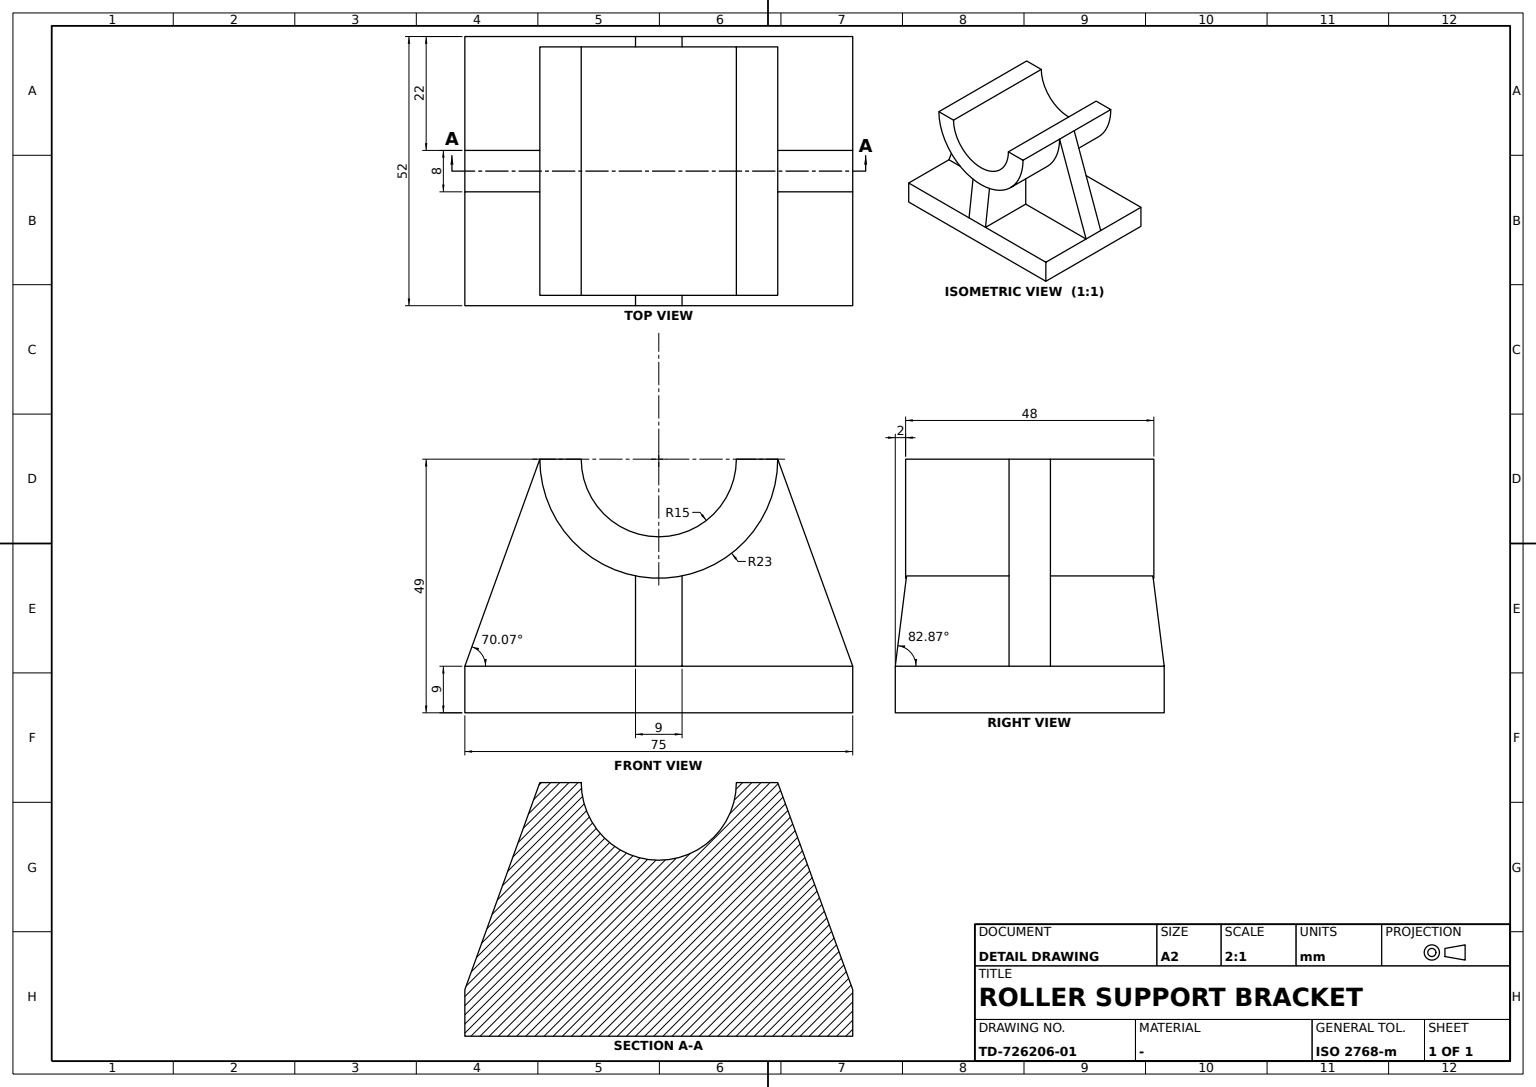
CATIA V5 part; units mm, degrees
sketch "Sketch1" plane through (0, 0, 0) normal (1, 0, 0) x (0, 1, 0)
  line L0 (37.5, 4.5) -> (37.5, -4.5)
  line L1 (37.5, -4.5) -> (-37.5, -4.5)
  line L2 (-37.5, -4.5) -> (-37.5, 4.5)
  line L3 (-37.5, 4.5) -> (37.5, 4.5)
  dimension "length L0" = 9
  dimension "length L1" = 75
  constraint vertical L0 y-axis
  constraint vertical L2 y-axis
  constraint horizontal L1 x-axis
  constraint horizontal L3 x-axis
  constraint equidistance L0 L2 origin
  constraint equidistance L1 L3 origin
extrude "Pad1" add sketch "Sketch1" along normal mid plane 52
sketch "Sketch2" plane through (0, 0, 0) normal (1, 0, 0) x (0, 1, 0)
  arc A0 (-23, 44.5) -> (23, 44.5) centre (0, 44.5) ccw
  point P0 (0, 44.5)
  point P1 (-23, 44.5)
  point P2 (23, 44.5)
  arc A1 (-15, 44.5) -> (15, 44.5) centre (0, 44.5) ccw
  line L0 (-23, 44.5) -> (-15, 44.5)
  line L1 (-37.5, -4.5) -> (37.5, -4.5) construction
  point P3 (-23, 44.5)
  point P4 (23, 44.5)
  point P5 (15, 44.5)
  line L2 (15, 44.5) -> (23, 44.5)
  dimension "radius A0" = 23
  dimension "radius A1" = 15
  dimension "distance L0 L1" = 49
  constraint coincidence P0 y-axis
  constraint coincidence P2 A0
  constraint coincidence P1 A0
  constraint coincidence P0 L0
  constraint coincidence L0 P5
  constraint coincidence L0 L2
  constraint coincidence P1 P3
  constraint coincidence P2 P4
  constraint horizontal L0 x-axis
  constraint horizontal L2 x-axis
extrude "Pad2" add sketch "Sketch2" along normal mid plane 48
sketch "Sketch3" plane through (0, 0, 0) normal (1, 0, 0) x (0, 1, 0)
  point P0 (23, 44.5)
  line L0 (23, 44.5) -> (37.5, 4.5)
  point P1 (37.5, 4.5)
  point P2 (23, 44.5)
  point P3 (37.5, 4.5)
  point P4 (-37.5, 4.5)
  point P5 (-23, 44.5)
  line L1 (-23, 44.5) -> (-37.5, 4.5)
  line L2 (37.5, 4.5) -> (-37.5, 4.5)
  point P6 (37.5, 4.5)
  point P7 (-37.5, 4.5)
  arc A0 (-23, 44.5) -> (23, 44.5) centre (0, 44.5) ccw
  point P8 (-23, 44.5)
  point P9 (23, 44.5)
  constraint coincidence P0 P2
  constraint coincidence P1 P3
  constraint coincidence P0 P9
  constraint coincidence P1 P6
  constraint coincidence P4 P7
  constraint coincidence P5 P8
  constraint symmetry P1 P4 y-axis
  constraint symmetry P0 P5 y-axis
  constraint symmetry L0 L1 y-axis
extrude "Pad3" add sketch "Sketch3" along normal mid plane 8
sketch "Sketch4" plane through (0, 0, 0) normal (0, 1, 0) x (-1, 0, 0)
  point P0 (-24, 20.5)
  line L0 (-24, 20.5) -> (-26, 4.5)
  point P1 (-26, 4.5)
  point P2 (-26, 4.5)
  line L1 (-24, 44.5) -> (-24, 21.5) construction
  dimension "D1" = 24
  constraint coincidence P1 P2
  constraint coincidence P0 L1
rib "Stiffener1" sketch "Sketch4" thickness 9 sides both
mirror "Mirror1" about plane through (0, 0, 0) normal (1, 0, 0) of "Stiffener1"
